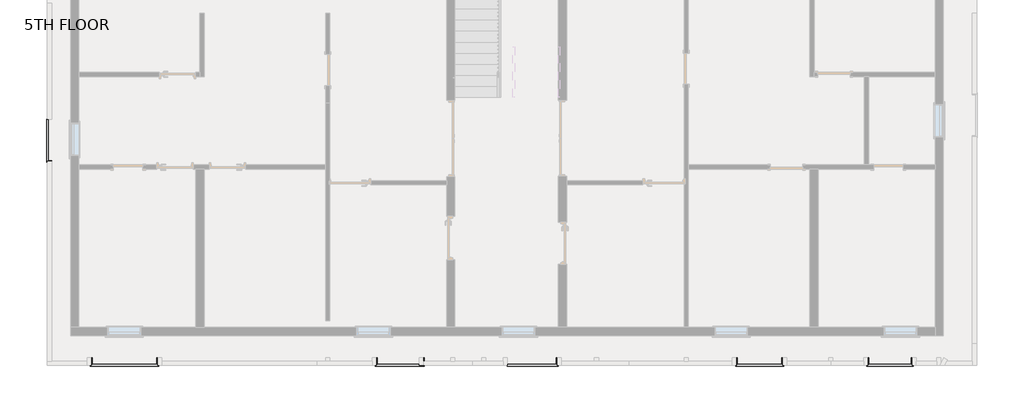
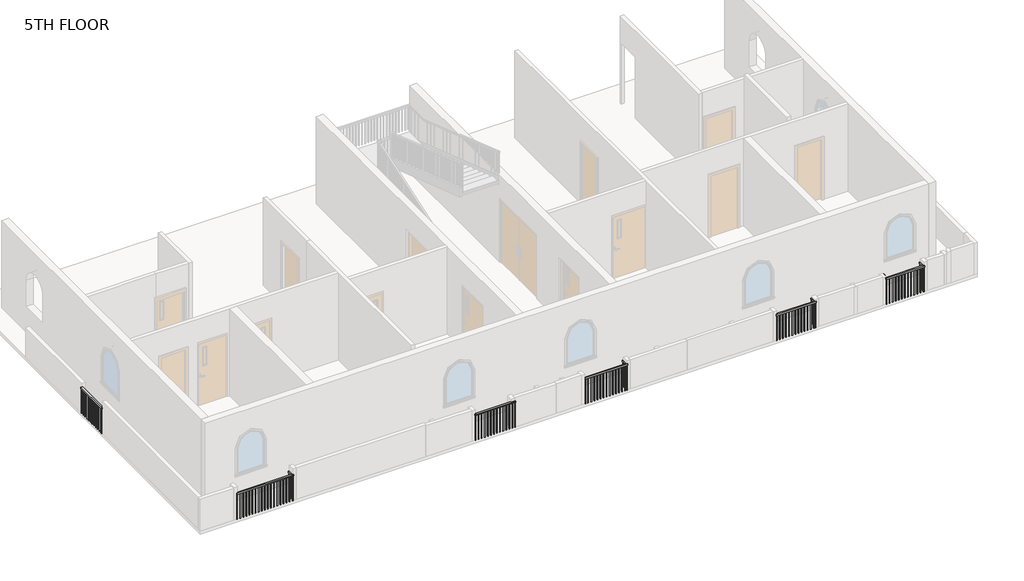
# One storey, part 3 of 7: 6 railings.
"""IFC4 building model written with IfcOpenShell, lengths in millimetres."""

from ifc_helpers import new_model, si_unit, frame, origin, place, context, project, spatial, polyline, outline, extrude, faceted_brep, element, save

model = new_model("IFC4")

# Units and contexts
model_context = context("Model", 3, world=origin())
ifc_project = project(units=[si_unit("LENGTHUNIT", "METRE", prefix="MILLI")], contexts=[model_context])

# Site, building, storey
site = spatial("IfcSite", under=ifc_project)
building = spatial("IfcBuilding", under=site)
storey = spatial("IfcBuildingStorey", under=building, Name="5TH FLOOR", Elevation=16002.0)

# Railings
placement = place(None, origin())
element("IfcRailing", 1, ObjectType="Handrail - Rectangular", at=placement, inside=storey, context=model_context, shape_type="SolidModel", body=[
    faceted_brep([(-11856.9067989, -4623.6932193, 16916.4), (-11856.9067989, -4623.6932193, 16865.6), (-11907.7067989, -4623.6932193, 16865.6), (-11907.7067989, -4623.6932193, 16916.4), (-11856.9067989, -4801.4932661, 16916.4), (-11856.9067989, -4801.4932661, 16865.6), (-11907.7067989, -4852.2932661, 16865.6), (-11907.7067989, -4852.2932661, 16916.4), (-10071.3470335, -4801.4932661, 16916.4), (-10071.3470335, -4801.4932661, 16865.6), (-10020.5470335, -4852.2932661, 16865.6), (-10020.5470335, -4852.2932661, 16916.4), (-10071.3470335, -4623.6932193, 16916.4), (-10020.5470335, -4623.6932193, 16916.4), (-10020.5470335, -4623.6932193, 16865.6), (-10071.3470335, -4623.6932193, 16865.6)], [[[0, 1, 2, 3]], [[1, 0, 4, 5]], [[2, 1, 5, 6]], [[3, 2, 6, 7]], [[0, 3, 7, 4]], [[5, 4, 8, 9]], [[6, 5, 9, 10]], [[7, 6, 10, 11]], [[4, 7, 11, 8]], [[12, 13, 14, 15]], [[9, 8, 12, 15]], [[10, 9, 15, 14]], [[11, 10, 14, 13]], [[8, 11, 13, 12]]]),
    extrude(outline(polyline([(-10036.4220335, -4633.2182661), (-10055.4720335, -4633.2182661), (-10055.4720335, -4614.1682661), (-10036.4220335, -4614.1682661), (-10036.4220335, -4633.2182661)])), frame((0.0, 0.0, 16002.0), z_axis=(0.0, 0.0, 1.0), x_axis=(1.0, 0.0, 0.0)), (0.0, 0.0, 1.0), 863.6),
    extrude(outline(polyline([(-10036.4220335, -4734.8182661), (-10055.4720335, -4734.8182661), (-10055.4720335, -4715.7682661), (-10036.4220335, -4715.7682661), (-10036.4220335, -4734.8182661)])), frame((0.0, 0.0, 16002.0), z_axis=(0.0, 0.0, 1.0), x_axis=(1.0, 0.0, 0.0)), (0.0, 0.0, 1.0), 863.6),
    extrude(outline(polyline([(-10063.0317989, -4836.4182661), (-10063.0317989, -4817.3682661), (-10043.9817989, -4817.3682661), (-10043.9817989, -4836.4182661), (-10063.0317989, -4836.4182661)])), frame((0.0, 0.0, 16002.0), z_axis=(0.0, 0.0, 1.0), x_axis=(1.0, 0.0, 0.0)), (0.0, 0.0, 1.0), 863.6),
    extrude(outline(polyline([(-10164.6317989, -4836.4182661), (-10164.6317989, -4817.3682661), (-10145.5817989, -4817.3682661), (-10145.5817989, -4836.4182661), (-10164.6317989, -4836.4182661)])), frame((0.0, 0.0, 16002.0), z_axis=(0.0, 0.0, 1.0), x_axis=(1.0, 0.0, 0.0)), (0.0, 0.0, 1.0), 863.6),
    extrude(outline(polyline([(-10266.2317989, -4836.4182661), (-10266.2317989, -4817.3682661), (-10247.1817989, -4817.3682661), (-10247.1817989, -4836.4182661), (-10266.2317989, -4836.4182661)])), frame((0.0, 0.0, 16002.0), z_axis=(0.0, 0.0, 1.0), x_axis=(1.0, 0.0, 0.0)), (0.0, 0.0, 1.0), 863.6),
    extrude(outline(polyline([(-10367.8317989, -4836.4182661), (-10367.8317989, -4817.3682661), (-10348.7817989, -4817.3682661), (-10348.7817989, -4836.4182661), (-10367.8317989, -4836.4182661)])), frame((0.0, 0.0, 16002.0), z_axis=(0.0, 0.0, 1.0), x_axis=(1.0, 0.0, 0.0)), (0.0, 0.0, 1.0), 863.6),
    extrude(outline(polyline([(-10469.4317989, -4836.4182661), (-10469.4317989, -4817.3682661), (-10450.3817989, -4817.3682661), (-10450.3817989, -4836.4182661), (-10469.4317989, -4836.4182661)])), frame((0.0, 0.0, 16002.0), z_axis=(0.0, 0.0, 1.0), x_axis=(1.0, 0.0, 0.0)), (0.0, 0.0, 1.0), 863.6),
    extrude(outline(polyline([(-10571.0317989, -4836.4182661), (-10571.0317989, -4817.3682661), (-10551.9817989, -4817.3682661), (-10551.9817989, -4836.4182661), (-10571.0317989, -4836.4182661)])), frame((0.0, 0.0, 16002.0), z_axis=(0.0, 0.0, 1.0), x_axis=(1.0, 0.0, 0.0)), (0.0, 0.0, 1.0), 863.6),
    extrude(outline(polyline([(-10672.6317989, -4836.4182661), (-10672.6317989, -4817.3682661), (-10653.5817989, -4817.3682661), (-10653.5817989, -4836.4182661), (-10672.6317989, -4836.4182661)])), frame((0.0, 0.0, 16002.0), z_axis=(0.0, 0.0, 1.0), x_axis=(1.0, 0.0, 0.0)), (0.0, 0.0, 1.0), 863.6),
    extrude(outline(polyline([(-10774.2317989, -4836.4182661), (-10774.2317989, -4817.3682661), (-10755.1817989, -4817.3682661), (-10755.1817989, -4836.4182661), (-10774.2317989, -4836.4182661)])), frame((0.0, 0.0, 16002.0), z_axis=(0.0, 0.0, 1.0), x_axis=(1.0, 0.0, 0.0)), (0.0, 0.0, 1.0), 863.6),
    extrude(outline(polyline([(-10875.8317989, -4836.4182661), (-10875.8317989, -4817.3682661), (-10856.7817989, -4817.3682661), (-10856.7817989, -4836.4182661), (-10875.8317989, -4836.4182661)])), frame((0.0, 0.0, 16002.0), z_axis=(0.0, 0.0, 1.0), x_axis=(1.0, 0.0, 0.0)), (0.0, 0.0, 1.0), 863.6),
    extrude(outline(polyline([(-10977.4317989, -4836.4182661), (-10977.4317989, -4817.3682661), (-10958.3817989, -4817.3682661), (-10958.3817989, -4836.4182661), (-10977.4317989, -4836.4182661)])), frame((0.0, 0.0, 16002.0), z_axis=(0.0, 0.0, 1.0), x_axis=(1.0, 0.0, 0.0)), (0.0, 0.0, 1.0), 863.6),
    extrude(outline(polyline([(-11079.0317989, -4836.4182661), (-11079.0317989, -4817.3682661), (-11059.9817989, -4817.3682661), (-11059.9817989, -4836.4182661), (-11079.0317989, -4836.4182661)])), frame((0.0, 0.0, 16002.0), z_axis=(0.0, 0.0, 1.0), x_axis=(1.0, 0.0, 0.0)), (0.0, 0.0, 1.0), 863.6),
    extrude(outline(polyline([(-11180.6317989, -4836.4182661), (-11180.6317989, -4817.3682661), (-11161.5817989, -4817.3682661), (-11161.5817989, -4836.4182661), (-11180.6317989, -4836.4182661)])), frame((0.0, 0.0, 16002.0), z_axis=(0.0, 0.0, 1.0), x_axis=(1.0, 0.0, 0.0)), (0.0, 0.0, 1.0), 863.6),
    extrude(outline(polyline([(-11282.2317989, -4836.4182661), (-11282.2317989, -4817.3682661), (-11263.1817989, -4817.3682661), (-11263.1817989, -4836.4182661), (-11282.2317989, -4836.4182661)])), frame((0.0, 0.0, 16002.0), z_axis=(0.0, 0.0, 1.0), x_axis=(1.0, 0.0, 0.0)), (0.0, 0.0, 1.0), 863.6),
    extrude(outline(polyline([(-11383.8317989, -4836.4182661), (-11383.8317989, -4817.3682661), (-11364.7817989, -4817.3682661), (-11364.7817989, -4836.4182661), (-11383.8317989, -4836.4182661)])), frame((0.0, 0.0, 16002.0), z_axis=(0.0, 0.0, 1.0), x_axis=(1.0, 0.0, 0.0)), (0.0, 0.0, 1.0), 863.6),
    extrude(outline(polyline([(-11485.4317989, -4836.4182661), (-11485.4317989, -4817.3682661), (-11466.3817989, -4817.3682661), (-11466.3817989, -4836.4182661), (-11485.4317989, -4836.4182661)])), frame((0.0, 0.0, 16002.0), z_axis=(0.0, 0.0, 1.0), x_axis=(1.0, 0.0, 0.0)), (0.0, 0.0, 1.0), 863.6),
    extrude(outline(polyline([(-11587.0317989, -4836.4182661), (-11587.0317989, -4817.3682661), (-11567.9817989, -4817.3682661), (-11567.9817989, -4836.4182661), (-11587.0317989, -4836.4182661)])), frame((0.0, 0.0, 16002.0), z_axis=(0.0, 0.0, 1.0), x_axis=(1.0, 0.0, 0.0)), (0.0, 0.0, 1.0), 863.6),
    extrude(outline(polyline([(-11688.6317989, -4836.4182661), (-11688.6317989, -4817.3682661), (-11669.5817989, -4817.3682661), (-11669.5817989, -4836.4182661), (-11688.6317989, -4836.4182661)])), frame((0.0, 0.0, 16002.0), z_axis=(0.0, 0.0, 1.0), x_axis=(1.0, 0.0, 0.0)), (0.0, 0.0, 1.0), 863.6),
    extrude(outline(polyline([(-11790.2317989, -4836.4182661), (-11790.2317989, -4817.3682661), (-11771.1817989, -4817.3682661), (-11771.1817989, -4836.4182661), (-11790.2317989, -4836.4182661)])), frame((0.0, 0.0, 16002.0), z_axis=(0.0, 0.0, 1.0), x_axis=(1.0, 0.0, 0.0)), (0.0, 0.0, 1.0), 863.6),
    extrude(outline(polyline([(-11891.8317989, -4817.3682193), (-11872.7817989, -4817.3682193), (-11872.7817989, -4836.4182193), (-11891.8317989, -4836.4182193), (-11891.8317989, -4817.3682193)])), frame((0.0, 0.0, 16002.0), z_axis=(0.0, 0.0, 1.0), x_axis=(1.0, 0.0, 0.0)), (0.0, 0.0, 1.0), 863.6),
    extrude(outline(polyline([(-11891.8317989, -4715.7682193), (-11872.7817989, -4715.7682193), (-11872.7817989, -4734.8182193), (-11891.8317989, -4734.8182193), (-11891.8317989, -4715.7682193)])), frame((0.0, 0.0, 16002.0), z_axis=(0.0, 0.0, 1.0), x_axis=(1.0, 0.0, 0.0)), (0.0, 0.0, 1.0), 863.6),
    extrude(outline(polyline([(-10055.4720335, -4836.4182661), (-10055.4720335, -4817.3682661), (-10036.4220335, -4817.3682661), (-10036.4220335, -4836.4182661), (-10055.4720335, -4836.4182661)])), frame((0.0, 0.0, 16002.0), z_axis=(0.0, 0.0, 1.0), x_axis=(1.0, 0.0, 0.0)), (0.0, 0.0, 1.0), 863.6),
    extrude(outline(polyline([(-11891.8317989, -4817.3682661), (-11872.7817989, -4817.3682661), (-11872.7817989, -4836.4182661), (-11891.8317989, -4836.4182661), (-11891.8317989, -4817.3682661)])), frame((0.0, 0.0, 16002.0), z_axis=(0.0, 0.0, 1.0), x_axis=(1.0, 0.0, 0.0)), (0.0, 0.0, 1.0), 863.6),
    extrude(outline(polyline([(-10036.4220335, -4642.7432193), (-10055.4720335, -4642.7432193), (-10055.4720335, -4623.6932193), (-10036.4220335, -4623.6932193), (-10036.4220335, -4642.7432193)])), frame((0.0, 0.0, 16002.0), z_axis=(0.0, 0.0, 1.0), x_axis=(1.0, 0.0, 0.0)), (0.0, 0.0, 1.0), 863.6),
    extrude(outline(polyline([(-11891.8317989, -4623.6932193), (-11872.7817989, -4623.6932193), (-11872.7817989, -4642.7432193), (-11891.8317989, -4642.7432193), (-11891.8317989, -4623.6932193)])), frame((0.0, 0.0, 16002.0), z_axis=(0.0, 0.0, 1.0), x_axis=(1.0, 0.0, 0.0)), (0.0, 0.0, 1.0), 863.6),
])
element("IfcRailing", 2, ObjectType="Handrail - Rectangular", at=placement, inside=storey, context=model_context, shape_type="SolidModel", body=[
    faceted_brep([(-3995.0987995, -4623.6932193, 16916.4), (-3995.0987995, -4623.6932193, 16865.6), (-4045.8987995, -4623.6932193, 16865.6), (-4045.8987995, -4623.6932193, 16916.4), (-3995.0987995, -4801.4932661, 16916.4), (-3995.0987995, -4801.4932661, 16865.6), (-4045.8987995, -4852.2932661, 16865.6), (-4045.8987995, -4852.2932661, 16916.4), (-2750.4987995, -4801.4932661, 16916.4), (-2750.4987995, -4801.4932661, 16865.6), (-2699.6987995, -4852.2932661, 16865.6), (-2699.6987995, -4852.2932661, 16916.4), (-2750.4987995, -4623.6932193, 16916.4), (-2699.6987995, -4623.6932193, 16916.4), (-2699.6987995, -4623.6932193, 16865.6), (-2750.4987995, -4623.6932193, 16865.6)], [[[0, 1, 2, 3]], [[1, 0, 4, 5]], [[2, 1, 5, 6]], [[3, 2, 6, 7]], [[0, 3, 7, 4]], [[5, 4, 8, 9]], [[6, 5, 9, 10]], [[7, 6, 10, 11]], [[4, 7, 11, 8]], [[12, 13, 14, 15]], [[9, 8, 12, 15]], [[10, 9, 15, 14]], [[11, 10, 14, 13]], [[8, 11, 13, 12]]]),
    extrude(outline(polyline([(-2715.5737995, -4633.2182661), (-2734.6237995, -4633.2182661), (-2734.6237995, -4614.1682661), (-2715.5737995, -4614.1682661), (-2715.5737995, -4633.2182661)])), frame((0.0, 0.0, 16002.0), z_axis=(0.0, 0.0, 1.0), x_axis=(1.0, 0.0, 0.0)), (0.0, 0.0, 1.0), 863.6),
    extrude(outline(polyline([(-2715.5737995, -4734.8182661), (-2734.6237995, -4734.8182661), (-2734.6237995, -4715.7682661), (-2715.5737995, -4715.7682661), (-2715.5737995, -4734.8182661)])), frame((0.0, 0.0, 16002.0), z_axis=(0.0, 0.0, 1.0), x_axis=(1.0, 0.0, 0.0)), (0.0, 0.0, 1.0), 863.6),
    extrude(outline(polyline([(-2810.8237995, -4836.4182661), (-2810.8237995, -4817.3682661), (-2791.7737995, -4817.3682661), (-2791.7737995, -4836.4182661), (-2810.8237995, -4836.4182661)])), frame((0.0, 0.0, 16002.0), z_axis=(0.0, 0.0, 1.0), x_axis=(1.0, 0.0, 0.0)), (0.0, 0.0, 1.0), 863.6),
    extrude(outline(polyline([(-2912.4237995, -4836.4182661), (-2912.4237995, -4817.3682661), (-2893.3737995, -4817.3682661), (-2893.3737995, -4836.4182661), (-2912.4237995, -4836.4182661)])), frame((0.0, 0.0, 16002.0), z_axis=(0.0, 0.0, 1.0), x_axis=(1.0, 0.0, 0.0)), (0.0, 0.0, 1.0), 863.6),
    extrude(outline(polyline([(-3014.0237995, -4836.4182661), (-3014.0237995, -4817.3682661), (-2994.9737995, -4817.3682661), (-2994.9737995, -4836.4182661), (-3014.0237995, -4836.4182661)])), frame((0.0, 0.0, 16002.0), z_axis=(0.0, 0.0, 1.0), x_axis=(1.0, 0.0, 0.0)), (0.0, 0.0, 1.0), 863.6),
    extrude(outline(polyline([(-3115.6237995, -4836.4182661), (-3115.6237995, -4817.3682661), (-3096.5737995, -4817.3682661), (-3096.5737995, -4836.4182661), (-3115.6237995, -4836.4182661)])), frame((0.0, 0.0, 16002.0), z_axis=(0.0, 0.0, 1.0), x_axis=(1.0, 0.0, 0.0)), (0.0, 0.0, 1.0), 863.6),
    extrude(outline(polyline([(-3217.2237995, -4836.4182661), (-3217.2237995, -4817.3682661), (-3198.1737995, -4817.3682661), (-3198.1737995, -4836.4182661), (-3217.2237995, -4836.4182661)])), frame((0.0, 0.0, 16002.0), z_axis=(0.0, 0.0, 1.0), x_axis=(1.0, 0.0, 0.0)), (0.0, 0.0, 1.0), 863.6),
    extrude(outline(polyline([(-3318.8237995, -4836.4182661), (-3318.8237995, -4817.3682661), (-3299.7737995, -4817.3682661), (-3299.7737995, -4836.4182661), (-3318.8237995, -4836.4182661)])), frame((0.0, 0.0, 16002.0), z_axis=(0.0, 0.0, 1.0), x_axis=(1.0, 0.0, 0.0)), (0.0, 0.0, 1.0), 863.6),
    extrude(outline(polyline([(-3420.4237995, -4836.4182661), (-3420.4237995, -4817.3682661), (-3401.3737995, -4817.3682661), (-3401.3737995, -4836.4182661), (-3420.4237995, -4836.4182661)])), frame((0.0, 0.0, 16002.0), z_axis=(0.0, 0.0, 1.0), x_axis=(1.0, 0.0, 0.0)), (0.0, 0.0, 1.0), 863.6),
    extrude(outline(polyline([(-3522.0237995, -4836.4182661), (-3522.0237995, -4817.3682661), (-3502.9737995, -4817.3682661), (-3502.9737995, -4836.4182661), (-3522.0237995, -4836.4182661)])), frame((0.0, 0.0, 16002.0), z_axis=(0.0, 0.0, 1.0), x_axis=(1.0, 0.0, 0.0)), (0.0, 0.0, 1.0), 863.6),
    extrude(outline(polyline([(-3623.6237995, -4836.4182661), (-3623.6237995, -4817.3682661), (-3604.5737995, -4817.3682661), (-3604.5737995, -4836.4182661), (-3623.6237995, -4836.4182661)])), frame((0.0, 0.0, 16002.0), z_axis=(0.0, 0.0, 1.0), x_axis=(1.0, 0.0, 0.0)), (0.0, 0.0, 1.0), 863.6),
    extrude(outline(polyline([(-3725.2237995, -4836.4182661), (-3725.2237995, -4817.3682661), (-3706.1737995, -4817.3682661), (-3706.1737995, -4836.4182661), (-3725.2237995, -4836.4182661)])), frame((0.0, 0.0, 16002.0), z_axis=(0.0, 0.0, 1.0), x_axis=(1.0, 0.0, 0.0)), (0.0, 0.0, 1.0), 863.6),
    extrude(outline(polyline([(-3826.8237995, -4836.4182661), (-3826.8237995, -4817.3682661), (-3807.7737995, -4817.3682661), (-3807.7737995, -4836.4182661), (-3826.8237995, -4836.4182661)])), frame((0.0, 0.0, 16002.0), z_axis=(0.0, 0.0, 1.0), x_axis=(1.0, 0.0, 0.0)), (0.0, 0.0, 1.0), 863.6),
    extrude(outline(polyline([(-3928.4237995, -4836.4182661), (-3928.4237995, -4817.3682661), (-3909.3737995, -4817.3682661), (-3909.3737995, -4836.4182661), (-3928.4237995, -4836.4182661)])), frame((0.0, 0.0, 16002.0), z_axis=(0.0, 0.0, 1.0), x_axis=(1.0, 0.0, 0.0)), (0.0, 0.0, 1.0), 863.6),
    extrude(outline(polyline([(-4030.0237995, -4817.3682193), (-4010.9737995, -4817.3682193), (-4010.9737995, -4836.4182193), (-4030.0237995, -4836.4182193), (-4030.0237995, -4817.3682193)])), frame((0.0, 0.0, 16002.0), z_axis=(0.0, 0.0, 1.0), x_axis=(1.0, 0.0, 0.0)), (0.0, 0.0, 1.0), 863.6),
    extrude(outline(polyline([(-4030.0237995, -4715.7682193), (-4010.9737995, -4715.7682193), (-4010.9737995, -4734.8182193), (-4030.0237995, -4734.8182193), (-4030.0237995, -4715.7682193)])), frame((0.0, 0.0, 16002.0), z_axis=(0.0, 0.0, 1.0), x_axis=(1.0, 0.0, 0.0)), (0.0, 0.0, 1.0), 863.6),
    extrude(outline(polyline([(-2734.6237995, -4836.4182661), (-2734.6237995, -4817.3682661), (-2715.5737995, -4817.3682661), (-2715.5737995, -4836.4182661), (-2734.6237995, -4836.4182661)])), frame((0.0, 0.0, 16002.0), z_axis=(0.0, 0.0, 1.0), x_axis=(1.0, 0.0, 0.0)), (0.0, 0.0, 1.0), 863.6),
    extrude(outline(polyline([(-4030.0237995, -4817.3682661), (-4010.9737995, -4817.3682661), (-4010.9737995, -4836.4182661), (-4030.0237995, -4836.4182661), (-4030.0237995, -4817.3682661)])), frame((0.0, 0.0, 16002.0), z_axis=(0.0, 0.0, 1.0), x_axis=(1.0, 0.0, 0.0)), (0.0, 0.0, 1.0), 863.6),
    extrude(outline(polyline([(-2715.5737995, -4642.7432193), (-2734.6237995, -4642.7432193), (-2734.6237995, -4623.6932193), (-2715.5737995, -4623.6932193), (-2715.5737995, -4642.7432193)])), frame((0.0, 0.0, 16002.0), z_axis=(0.0, 0.0, 1.0), x_axis=(1.0, 0.0, 0.0)), (0.0, 0.0, 1.0), 863.6),
    extrude(outline(polyline([(-4030.0237995, -4623.6932193), (-4010.9737995, -4623.6932193), (-4010.9737995, -4642.7432193), (-4030.0237995, -4642.7432193), (-4030.0237995, -4623.6932193)])), frame((0.0, 0.0, 16002.0), z_axis=(0.0, 0.0, 1.0), x_axis=(1.0, 0.0, 0.0)), (0.0, 0.0, 1.0), 863.6),
])
element("IfcRailing", 3, ObjectType="Handrail - Rectangular", at=placement, inside=storey, context=model_context, shape_type="SolidModel", body=[
    faceted_brep([(-406.2065315, -4801.4932661, 16916.4), (-406.2065315, -4801.4932661, 16865.6), (-406.2065315, -4852.2932661, 16865.6), (-406.2065315, -4852.2932661, 16916.4), (944.6932011, -4801.4932661, 16916.4), (944.6932011, -4801.4932661, 16865.6), (995.4932011, -4852.2932661, 16865.6), (995.4932011, -4852.2932661, 16916.4), (944.6932011, -4623.6932193, 16916.4), (995.4932011, -4623.6932193, 16916.4), (995.4932011, -4623.6932193, 16865.6), (944.6932011, -4623.6932193, 16865.6)], [[[0, 1, 2, 3]], [[1, 0, 4, 5]], [[2, 1, 5, 6]], [[3, 2, 6, 7]], [[0, 3, 7, 4]], [[8, 9, 10, 11]], [[5, 4, 8, 11]], [[6, 5, 11, 10]], [[7, 6, 10, 9]], [[4, 7, 9, 8]]]),
    extrude(outline(polyline([(979.6182011, -4633.2182661), (960.5682011, -4633.2182661), (960.5682011, -4614.1682661), (979.6182011, -4614.1682661), (979.6182011, -4633.2182661)])), frame((0.0, 0.0, 16002.0), z_axis=(0.0, 0.0, 1.0), x_axis=(1.0, 0.0, 0.0)), (0.0, 0.0, 1.0), 863.6),
    extrude(outline(polyline([(979.6182011, -4734.8182661), (960.5682011, -4734.8182661), (960.5682011, -4715.7682661), (979.6182011, -4715.7682661), (979.6182011, -4734.8182661)])), frame((0.0, 0.0, 16002.0), z_axis=(0.0, 0.0, 1.0), x_axis=(1.0, 0.0, 0.0)), (0.0, 0.0, 1.0), 863.6),
    extrude(outline(polyline([(905.0684685, -4836.4182661), (905.0684685, -4817.3682661), (924.1184685, -4817.3682661), (924.1184685, -4836.4182661), (905.0684685, -4836.4182661)])), frame((0.0, 0.0, 16002.0), z_axis=(0.0, 0.0, 1.0), x_axis=(1.0, 0.0, 0.0)), (0.0, 0.0, 1.0), 863.6),
    extrude(outline(polyline([(803.4684685, -4836.4182661), (803.4684685, -4817.3682661), (822.5184685, -4817.3682661), (822.5184685, -4836.4182661), (803.4684685, -4836.4182661)])), frame((0.0, 0.0, 16002.0), z_axis=(0.0, 0.0, 1.0), x_axis=(1.0, 0.0, 0.0)), (0.0, 0.0, 1.0), 863.6),
    extrude(outline(polyline([(701.8684685, -4836.4182661), (701.8684685, -4817.3682661), (720.9184685, -4817.3682661), (720.9184685, -4836.4182661), (701.8684685, -4836.4182661)])), frame((0.0, 0.0, 16002.0), z_axis=(0.0, 0.0, 1.0), x_axis=(1.0, 0.0, 0.0)), (0.0, 0.0, 1.0), 863.6),
    extrude(outline(polyline([(600.2684685, -4836.4182661), (600.2684685, -4817.3682661), (619.3184685, -4817.3682661), (619.3184685, -4836.4182661), (600.2684685, -4836.4182661)])), frame((0.0, 0.0, 16002.0), z_axis=(0.0, 0.0, 1.0), x_axis=(1.0, 0.0, 0.0)), (0.0, 0.0, 1.0), 863.6),
    extrude(outline(polyline([(498.6684685, -4836.4182661), (498.6684685, -4817.3682661), (517.7184685, -4817.3682661), (517.7184685, -4836.4182661), (498.6684685, -4836.4182661)])), frame((0.0, 0.0, 16002.0), z_axis=(0.0, 0.0, 1.0), x_axis=(1.0, 0.0, 0.0)), (0.0, 0.0, 1.0), 863.6),
    extrude(outline(polyline([(397.0684685, -4836.4182661), (397.0684685, -4817.3682661), (416.1184685, -4817.3682661), (416.1184685, -4836.4182661), (397.0684685, -4836.4182661)])), frame((0.0, 0.0, 16002.0), z_axis=(0.0, 0.0, 1.0), x_axis=(1.0, 0.0, 0.0)), (0.0, 0.0, 1.0), 863.6),
    extrude(outline(polyline([(295.4684685, -4836.4182661), (295.4684685, -4817.3682661), (314.5184685, -4817.3682661), (314.5184685, -4836.4182661), (295.4684685, -4836.4182661)])), frame((0.0, 0.0, 16002.0), z_axis=(0.0, 0.0, 1.0), x_axis=(1.0, 0.0, 0.0)), (0.0, 0.0, 1.0), 863.6),
    extrude(outline(polyline([(193.8684685, -4836.4182661), (193.8684685, -4817.3682661), (212.9184685, -4817.3682661), (212.9184685, -4836.4182661), (193.8684685, -4836.4182661)])), frame((0.0, 0.0, 16002.0), z_axis=(0.0, 0.0, 1.0), x_axis=(1.0, 0.0, 0.0)), (0.0, 0.0, 1.0), 863.6),
    extrude(outline(polyline([(92.2684685, -4836.4182661), (92.2684685, -4817.3682661), (111.3184685, -4817.3682661), (111.3184685, -4836.4182661), (92.2684685, -4836.4182661)])), frame((0.0, 0.0, 16002.0), z_axis=(0.0, 0.0, 1.0), x_axis=(1.0, 0.0, 0.0)), (0.0, 0.0, 1.0), 863.6),
    extrude(outline(polyline([(-9.3315315, -4836.4182661), (-9.3315315, -4817.3682661), (9.7184685, -4817.3682661), (9.7184685, -4836.4182661), (-9.3315315, -4836.4182661)])), frame((0.0, 0.0, 16002.0), z_axis=(0.0, 0.0, 1.0), x_axis=(1.0, 0.0, 0.0)), (0.0, 0.0, 1.0), 863.6),
    extrude(outline(polyline([(-110.9315315, -4836.4182661), (-110.9315315, -4817.3682661), (-91.8815315, -4817.3682661), (-91.8815315, -4836.4182661), (-110.9315315, -4836.4182661)])), frame((0.0, 0.0, 16002.0), z_axis=(0.0, 0.0, 1.0), x_axis=(1.0, 0.0, 0.0)), (0.0, 0.0, 1.0), 863.6),
    extrude(outline(polyline([(-212.5315315, -4836.4182661), (-212.5315315, -4817.3682661), (-193.4815315, -4817.3682661), (-193.4815315, -4836.4182661), (-212.5315315, -4836.4182661)])), frame((0.0, 0.0, 16002.0), z_axis=(0.0, 0.0, 1.0), x_axis=(1.0, 0.0, 0.0)), (0.0, 0.0, 1.0), 863.6),
    extrude(outline(polyline([(-314.1315315, -4836.4182661), (-314.1315315, -4817.3682661), (-295.0815315, -4817.3682661), (-295.0815315, -4836.4182661), (-314.1315315, -4836.4182661)])), frame((0.0, 0.0, 16002.0), z_axis=(0.0, 0.0, 1.0), x_axis=(1.0, 0.0, 0.0)), (0.0, 0.0, 1.0), 863.6),
    extrude(outline(polyline([(960.5682011, -4836.4182661), (960.5682011, -4817.3682661), (979.6182011, -4817.3682661), (979.6182011, -4836.4182661), (960.5682011, -4836.4182661)])), frame((0.0, 0.0, 16002.0), z_axis=(0.0, 0.0, 1.0), x_axis=(1.0, 0.0, 0.0)), (0.0, 0.0, 1.0), 863.6),
    extrude(outline(polyline([(979.6182011, -4642.7432193), (960.5682011, -4642.7432193), (960.5682011, -4623.6932193), (979.6182011, -4623.6932193), (979.6182011, -4642.7432193)])), frame((0.0, 0.0, 16002.0), z_axis=(0.0, 0.0, 1.0), x_axis=(1.0, 0.0, 0.0)), (0.0, 0.0, 1.0), 863.6),
    extrude(outline(polyline([(-406.2065315, -4836.4182661), (-406.2065315, -4817.3682661), (-387.1565315, -4817.3682661), (-387.1565315, -4836.4182661), (-406.2065315, -4836.4182661)])), frame((0.0, 0.0, 16002.0), z_axis=(0.0, 0.0, 1.0), x_axis=(1.0, 0.0, 0.0)), (0.0, 0.0, 1.0), 863.6),
])
element("IfcRailing", 4, ObjectType="Handrail - Rectangular", at=placement, inside=storey, context=model_context, shape_type="SolidModel", body=[
    faceted_brep([(5942.6512082, -4623.6932193, 16916.4), (5942.6512082, -4623.6932193, 16865.6), (5891.8512082, -4623.6932193, 16865.6), (5891.8512082, -4623.6932193, 16916.4), (5942.6512082, -4801.4932661, 16916.4), (5942.6512082, -4801.4932661, 16865.6), (5891.8512082, -4852.2932661, 16865.6), (5891.8512082, -4852.2932661, 16916.4), (7164.9011643, -4801.4932661, 16916.4), (7164.9011643, -4801.4932661, 16865.6), (7215.7011643, -4852.2932661, 16865.6), (7215.7011643, -4852.2932661, 16916.4), (7164.9011643, -4623.6932193, 16916.4), (7215.7011643, -4623.6932193, 16916.4), (7215.7011643, -4623.6932193, 16865.6), (7164.9011643, -4623.6932193, 16865.6)], [[[0, 1, 2, 3]], [[1, 0, 4, 5]], [[2, 1, 5, 6]], [[3, 2, 6, 7]], [[0, 3, 7, 4]], [[5, 4, 8, 9]], [[6, 5, 9, 10]], [[7, 6, 10, 11]], [[4, 7, 11, 8]], [[12, 13, 14, 15]], [[9, 8, 12, 15]], [[10, 9, 15, 14]], [[11, 10, 14, 13]], [[8, 11, 13, 12]]]),
    extrude(outline(polyline([(7199.8261643, -4633.2182661), (7180.7761643, -4633.2182661), (7180.7761643, -4614.1682661), (7199.8261643, -4614.1682661), (7199.8261643, -4633.2182661)])), frame((0.0, 0.0, 16002.0), z_axis=(0.0, 0.0, 1.0), x_axis=(1.0, 0.0, 0.0)), (0.0, 0.0, 1.0), 863.6),
    extrude(outline(polyline([(7199.8261643, -4734.8182661), (7180.7761643, -4734.8182661), (7180.7761643, -4715.7682661), (7199.8261643, -4715.7682661), (7199.8261643, -4734.8182661)])), frame((0.0, 0.0, 16002.0), z_axis=(0.0, 0.0, 1.0), x_axis=(1.0, 0.0, 0.0)), (0.0, 0.0, 1.0), 863.6),
    extrude(outline(polyline([(7126.9262082, -4836.4182661), (7126.9262082, -4817.3682661), (7145.9762082, -4817.3682661), (7145.9762082, -4836.4182661), (7126.9262082, -4836.4182661)])), frame((0.0, 0.0, 16002.0), z_axis=(0.0, 0.0, 1.0), x_axis=(1.0, 0.0, 0.0)), (0.0, 0.0, 1.0), 863.6),
    extrude(outline(polyline([(7025.3262082, -4836.4182661), (7025.3262082, -4817.3682661), (7044.3762082, -4817.3682661), (7044.3762082, -4836.4182661), (7025.3262082, -4836.4182661)])), frame((0.0, 0.0, 16002.0), z_axis=(0.0, 0.0, 1.0), x_axis=(1.0, 0.0, 0.0)), (0.0, 0.0, 1.0), 863.6),
    extrude(outline(polyline([(6923.7262082, -4836.4182661), (6923.7262082, -4817.3682661), (6942.7762082, -4817.3682661), (6942.7762082, -4836.4182661), (6923.7262082, -4836.4182661)])), frame((0.0, 0.0, 16002.0), z_axis=(0.0, 0.0, 1.0), x_axis=(1.0, 0.0, 0.0)), (0.0, 0.0, 1.0), 863.6),
    extrude(outline(polyline([(6822.1262082, -4836.4182661), (6822.1262082, -4817.3682661), (6841.1762082, -4817.3682661), (6841.1762082, -4836.4182661), (6822.1262082, -4836.4182661)])), frame((0.0, 0.0, 16002.0), z_axis=(0.0, 0.0, 1.0), x_axis=(1.0, 0.0, 0.0)), (0.0, 0.0, 1.0), 863.6),
    extrude(outline(polyline([(6720.5262082, -4836.4182661), (6720.5262082, -4817.3682661), (6739.5762082, -4817.3682661), (6739.5762082, -4836.4182661), (6720.5262082, -4836.4182661)])), frame((0.0, 0.0, 16002.0), z_axis=(0.0, 0.0, 1.0), x_axis=(1.0, 0.0, 0.0)), (0.0, 0.0, 1.0), 863.6),
    extrude(outline(polyline([(6618.9262082, -4836.4182661), (6618.9262082, -4817.3682661), (6637.9762082, -4817.3682661), (6637.9762082, -4836.4182661), (6618.9262082, -4836.4182661)])), frame((0.0, 0.0, 16002.0), z_axis=(0.0, 0.0, 1.0), x_axis=(1.0, 0.0, 0.0)), (0.0, 0.0, 1.0), 863.6),
    extrude(outline(polyline([(6517.3262082, -4836.4182661), (6517.3262082, -4817.3682661), (6536.3762082, -4817.3682661), (6536.3762082, -4836.4182661), (6517.3262082, -4836.4182661)])), frame((0.0, 0.0, 16002.0), z_axis=(0.0, 0.0, 1.0), x_axis=(1.0, 0.0, 0.0)), (0.0, 0.0, 1.0), 863.6),
    extrude(outline(polyline([(6415.7262082, -4836.4182661), (6415.7262082, -4817.3682661), (6434.7762082, -4817.3682661), (6434.7762082, -4836.4182661), (6415.7262082, -4836.4182661)])), frame((0.0, 0.0, 16002.0), z_axis=(0.0, 0.0, 1.0), x_axis=(1.0, 0.0, 0.0)), (0.0, 0.0, 1.0), 863.6),
    extrude(outline(polyline([(6314.1262082, -4836.4182661), (6314.1262082, -4817.3682661), (6333.1762082, -4817.3682661), (6333.1762082, -4836.4182661), (6314.1262082, -4836.4182661)])), frame((0.0, 0.0, 16002.0), z_axis=(0.0, 0.0, 1.0), x_axis=(1.0, 0.0, 0.0)), (0.0, 0.0, 1.0), 863.6),
    extrude(outline(polyline([(6212.5262082, -4836.4182661), (6212.5262082, -4817.3682661), (6231.5762082, -4817.3682661), (6231.5762082, -4836.4182661), (6212.5262082, -4836.4182661)])), frame((0.0, 0.0, 16002.0), z_axis=(0.0, 0.0, 1.0), x_axis=(1.0, 0.0, 0.0)), (0.0, 0.0, 1.0), 863.6),
    extrude(outline(polyline([(6110.9262082, -4836.4182661), (6110.9262082, -4817.3682661), (6129.9762082, -4817.3682661), (6129.9762082, -4836.4182661), (6110.9262082, -4836.4182661)])), frame((0.0, 0.0, 16002.0), z_axis=(0.0, 0.0, 1.0), x_axis=(1.0, 0.0, 0.0)), (0.0, 0.0, 1.0), 863.6),
    extrude(outline(polyline([(6009.3262082, -4836.4182661), (6009.3262082, -4817.3682661), (6028.3762082, -4817.3682661), (6028.3762082, -4836.4182661), (6009.3262082, -4836.4182661)])), frame((0.0, 0.0, 16002.0), z_axis=(0.0, 0.0, 1.0), x_axis=(1.0, 0.0, 0.0)), (0.0, 0.0, 1.0), 863.6),
    extrude(outline(polyline([(5907.7262082, -4817.3682193), (5926.7762082, -4817.3682193), (5926.7762082, -4836.4182193), (5907.7262082, -4836.4182193), (5907.7262082, -4817.3682193)])), frame((0.0, 0.0, 16002.0), z_axis=(0.0, 0.0, 1.0), x_axis=(1.0, 0.0, 0.0)), (0.0, 0.0, 1.0), 863.6),
    extrude(outline(polyline([(5907.7262082, -4715.7682193), (5926.7762082, -4715.7682193), (5926.7762082, -4734.8182193), (5907.7262082, -4734.8182193), (5907.7262082, -4715.7682193)])), frame((0.0, 0.0, 16002.0), z_axis=(0.0, 0.0, 1.0), x_axis=(1.0, 0.0, 0.0)), (0.0, 0.0, 1.0), 863.6),
    extrude(outline(polyline([(7180.7761643, -4836.4182661), (7180.7761643, -4817.3682661), (7199.8261643, -4817.3682661), (7199.8261643, -4836.4182661), (7180.7761643, -4836.4182661)])), frame((0.0, 0.0, 16002.0), z_axis=(0.0, 0.0, 1.0), x_axis=(1.0, 0.0, 0.0)), (0.0, 0.0, 1.0), 863.6),
    extrude(outline(polyline([(5907.7262082, -4817.3682661), (5926.7762082, -4817.3682661), (5926.7762082, -4836.4182661), (5907.7262082, -4836.4182661), (5907.7262082, -4817.3682661)])), frame((0.0, 0.0, 16002.0), z_axis=(0.0, 0.0, 1.0), x_axis=(1.0, 0.0, 0.0)), (0.0, 0.0, 1.0), 863.6),
    extrude(outline(polyline([(7199.8261643, -4642.7432193), (7180.7761643, -4642.7432193), (7180.7761643, -4623.6932193), (7199.8261643, -4623.6932193), (7199.8261643, -4642.7432193)])), frame((0.0, 0.0, 16002.0), z_axis=(0.0, 0.0, 1.0), x_axis=(1.0, 0.0, 0.0)), (0.0, 0.0, 1.0), 863.6),
    extrude(outline(polyline([(5907.7262082, -4623.6932193), (5926.7762082, -4623.6932193), (5926.7762082, -4642.7432193), (5907.7262082, -4642.7432193), (5907.7262082, -4623.6932193)])), frame((0.0, 0.0, 16002.0), z_axis=(0.0, 0.0, 1.0), x_axis=(1.0, 0.0, 0.0)), (0.0, 0.0, 1.0), 863.6),
])
element("IfcRailing", 5, ObjectType="Handrail - Rectangular", at=placement, inside=storey, context=model_context, shape_type="SolidModel", body=[
    faceted_brep([(9562.1512082, -4623.6932193, 16916.4), (9562.1512082, -4623.6932193, 16865.6), (9511.3512082, -4623.6932193, 16865.6), (9511.3512082, -4623.6932193, 16916.4), (9562.1512082, -4801.4932661, 16916.4), (9562.1512082, -4801.4932661, 16865.6), (9511.3512082, -4852.2932661, 16865.6), (9511.3512082, -4852.2932661, 16916.4), (10738.7617205, -4801.4932661, 16916.4), (10738.7617205, -4801.4932661, 16865.6), (10789.5617205, -4852.2932661, 16865.6), (10789.5617205, -4852.2932661, 16916.4), (10738.7617205, -4623.6932193, 16916.4), (10789.5617205, -4623.6932193, 16916.4), (10789.5617205, -4623.6932193, 16865.6), (10738.7617205, -4623.6932193, 16865.6)], [[[0, 1, 2, 3]], [[1, 0, 4, 5]], [[2, 1, 5, 6]], [[3, 2, 6, 7]], [[0, 3, 7, 4]], [[5, 4, 8, 9]], [[6, 5, 9, 10]], [[7, 6, 10, 11]], [[4, 7, 11, 8]], [[12, 13, 14, 15]], [[9, 8, 12, 15]], [[10, 9, 15, 14]], [[11, 10, 14, 13]], [[8, 11, 13, 12]]]),
    extrude(outline(polyline([(10754.6367205, -4633.2182661), (10754.6367205, -4614.1682661), (10773.6867205, -4614.1682661), (10773.6867205, -4633.2182661), (10754.6367205, -4633.2182661)])), frame((0.0, 0.0, 16002.0), z_axis=(0.0, 0.0, 1.0), x_axis=(1.0, 0.0, 0.0)), (0.0, 0.0, 1.0), 863.6),
    extrude(outline(polyline([(10754.6367205, -4734.8182661), (10754.6367205, -4715.7682661), (10773.6867205, -4715.7682661), (10773.6867205, -4734.8182661), (10754.6367205, -4734.8182661)])), frame((0.0, 0.0, 16002.0), z_axis=(0.0, 0.0, 1.0), x_axis=(1.0, 0.0, 0.0)), (0.0, 0.0, 1.0), 863.6),
    extrude(outline(polyline([(10746.4262082, -4817.3682661), (10765.4762082, -4817.3682661), (10765.4762082, -4836.4182661), (10746.4262082, -4836.4182661), (10746.4262082, -4817.3682661)])), frame((0.0, 0.0, 16002.0), z_axis=(0.0, 0.0, 1.0), x_axis=(1.0, 0.0, 0.0)), (0.0, 0.0, 1.0), 863.6),
    extrude(outline(polyline([(10644.8262082, -4817.3682661), (10663.8762082, -4817.3682661), (10663.8762082, -4836.4182661), (10644.8262082, -4836.4182661), (10644.8262082, -4817.3682661)])), frame((0.0, 0.0, 16002.0), z_axis=(0.0, 0.0, 1.0), x_axis=(1.0, 0.0, 0.0)), (0.0, 0.0, 1.0), 863.6),
    extrude(outline(polyline([(10543.2262082, -4817.3682661), (10562.2762082, -4817.3682661), (10562.2762082, -4836.4182661), (10543.2262082, -4836.4182661), (10543.2262082, -4817.3682661)])), frame((0.0, 0.0, 16002.0), z_axis=(0.0, 0.0, 1.0), x_axis=(1.0, 0.0, 0.0)), (0.0, 0.0, 1.0), 863.6),
    extrude(outline(polyline([(10441.6262082, -4817.3682661), (10460.6762082, -4817.3682661), (10460.6762082, -4836.4182661), (10441.6262082, -4836.4182661), (10441.6262082, -4817.3682661)])), frame((0.0, 0.0, 16002.0), z_axis=(0.0, 0.0, 1.0), x_axis=(1.0, 0.0, 0.0)), (0.0, 0.0, 1.0), 863.6),
    extrude(outline(polyline([(10340.0262082, -4817.3682661), (10359.0762082, -4817.3682661), (10359.0762082, -4836.4182661), (10340.0262082, -4836.4182661), (10340.0262082, -4817.3682661)])), frame((0.0, 0.0, 16002.0), z_axis=(0.0, 0.0, 1.0), x_axis=(1.0, 0.0, 0.0)), (0.0, 0.0, 1.0), 863.6),
    extrude(outline(polyline([(10238.4262082, -4817.3682661), (10257.4762082, -4817.3682661), (10257.4762082, -4836.4182661), (10238.4262082, -4836.4182661), (10238.4262082, -4817.3682661)])), frame((0.0, 0.0, 16002.0), z_axis=(0.0, 0.0, 1.0), x_axis=(1.0, 0.0, 0.0)), (0.0, 0.0, 1.0), 863.6),
    extrude(outline(polyline([(10136.8262082, -4817.3682661), (10155.8762082, -4817.3682661), (10155.8762082, -4836.4182661), (10136.8262082, -4836.4182661), (10136.8262082, -4817.3682661)])), frame((0.0, 0.0, 16002.0), z_axis=(0.0, 0.0, 1.0), x_axis=(1.0, 0.0, 0.0)), (0.0, 0.0, 1.0), 863.6),
    extrude(outline(polyline([(10035.2262082, -4817.3682661), (10054.2762082, -4817.3682661), (10054.2762082, -4836.4182661), (10035.2262082, -4836.4182661), (10035.2262082, -4817.3682661)])), frame((0.0, 0.0, 16002.0), z_axis=(0.0, 0.0, 1.0), x_axis=(1.0, 0.0, 0.0)), (0.0, 0.0, 1.0), 863.6),
    extrude(outline(polyline([(9933.6262082, -4817.3682661), (9952.6762082, -4817.3682661), (9952.6762082, -4836.4182661), (9933.6262082, -4836.4182661), (9933.6262082, -4817.3682661)])), frame((0.0, 0.0, 16002.0), z_axis=(0.0, 0.0, 1.0), x_axis=(1.0, 0.0, 0.0)), (0.0, 0.0, 1.0), 863.6),
    extrude(outline(polyline([(9832.0262082, -4817.3682661), (9851.0762082, -4817.3682661), (9851.0762082, -4836.4182661), (9832.0262082, -4836.4182661), (9832.0262082, -4817.3682661)])), frame((0.0, 0.0, 16002.0), z_axis=(0.0, 0.0, 1.0), x_axis=(1.0, 0.0, 0.0)), (0.0, 0.0, 1.0), 863.6),
    extrude(outline(polyline([(9730.4262082, -4817.3682661), (9749.4762082, -4817.3682661), (9749.4762082, -4836.4182661), (9730.4262082, -4836.4182661), (9730.4262082, -4817.3682661)])), frame((0.0, 0.0, 16002.0), z_axis=(0.0, 0.0, 1.0), x_axis=(1.0, 0.0, 0.0)), (0.0, 0.0, 1.0), 863.6),
    extrude(outline(polyline([(9628.8262082, -4817.3682661), (9647.8762082, -4817.3682661), (9647.8762082, -4836.4182661), (9628.8262082, -4836.4182661), (9628.8262082, -4817.3682661)])), frame((0.0, 0.0, 16002.0), z_axis=(0.0, 0.0, 1.0), x_axis=(1.0, 0.0, 0.0)), (0.0, 0.0, 1.0), 863.6),
    extrude(outline(polyline([(9546.2762082, -4817.3682193), (9546.2762082, -4836.4182193), (9527.2262082, -4836.4182193), (9527.2262082, -4817.3682193), (9546.2762082, -4817.3682193)])), frame((0.0, 0.0, 16002.0), z_axis=(0.0, 0.0, 1.0), x_axis=(1.0, 0.0, 0.0)), (0.0, 0.0, 1.0), 863.6),
    extrude(outline(polyline([(9546.2762082, -4715.7682193), (9546.2762082, -4734.8182193), (9527.2262082, -4734.8182193), (9527.2262082, -4715.7682193), (9546.2762082, -4715.7682193)])), frame((0.0, 0.0, 16002.0), z_axis=(0.0, 0.0, 1.0), x_axis=(1.0, 0.0, 0.0)), (0.0, 0.0, 1.0), 863.6),
    extrude(outline(polyline([(10754.6367205, -4817.3682661), (10773.6867205, -4817.3682661), (10773.6867205, -4836.4182661), (10754.6367205, -4836.4182661), (10754.6367205, -4817.3682661)])), frame((0.0, 0.0, 16002.0), z_axis=(0.0, 0.0, 1.0), x_axis=(1.0, 0.0, 0.0)), (0.0, 0.0, 1.0), 863.6),
    extrude(outline(polyline([(9546.2762082, -4817.3682661), (9546.2762082, -4836.4182661), (9527.2262082, -4836.4182661), (9527.2262082, -4817.3682661), (9546.2762082, -4817.3682661)])), frame((0.0, 0.0, 16002.0), z_axis=(0.0, 0.0, 1.0), x_axis=(1.0, 0.0, 0.0)), (0.0, 0.0, 1.0), 863.6),
    extrude(outline(polyline([(10754.6367205, -4642.7432193), (10754.6367205, -4623.6932193), (10773.6867205, -4623.6932193), (10773.6867205, -4642.7432193), (10754.6367205, -4642.7432193)])), frame((0.0, 0.0, 16002.0), z_axis=(0.0, 0.0, 1.0), x_axis=(1.0, 0.0, 0.0)), (0.0, 0.0, 1.0), 863.6),
    extrude(outline(polyline([(9546.2762082, -4623.6932193), (9546.2762082, -4642.7432193), (9527.2262082, -4642.7432193), (9527.2262082, -4623.6932193), (9546.2762082, -4623.6932193)])), frame((0.0, 0.0, 16002.0), z_axis=(0.0, 0.0, 1.0), x_axis=(1.0, 0.0, 0.0)), (0.0, 0.0, 1.0), 863.6),
])
element("IfcRailing", 6, ObjectType="Handrail - Rectangular", at=placement, inside=storey, context=model_context, shape_type="SolidModel", body=[
    faceted_brep([(-13063.4067989, 1953.9604213, 16916.4), (-13063.4067989, 1953.9604213, 16865.6), (-13114.2067989, 1953.9604213, 16865.6), (-13114.2067989, 1953.9604213, 16916.4), (-13063.4067989, 818.2567339, 16916.4), (-13063.4067989, 818.2567339, 16865.6), (-13114.2067989, 767.4567339, 16865.6), (-13114.2067989, 767.4567339, 16916.4), (-12974.5067989, 818.2567339, 16916.4), (-12974.5067989, 767.4567339, 16916.4), (-12974.5067989, 767.4567339, 16865.6), (-12974.5067989, 818.2567339, 16865.6)], [[[0, 1, 2, 3]], [[1, 0, 4, 5]], [[2, 1, 5, 6]], [[3, 2, 6, 7]], [[0, 3, 7, 4]], [[8, 9, 10, 11]], [[5, 4, 8, 11]], [[6, 5, 11, 10]], [[7, 6, 10, 9]], [[4, 7, 9, 8]]]),
    extrude(outline(polyline([(-12996.7317989, 783.3317339), (-12996.7317989, 802.3817339), (-12977.6817989, 802.3817339), (-12977.6817989, 783.3317339), (-12996.7317989, 783.3317339)])), frame((0.0, 0.0, 16002.0), z_axis=(0.0, 0.0, 1.0), x_axis=(1.0, 0.0, 0.0)), (0.0, 0.0, 1.0), 863.6),
    extrude(outline(polyline([(-13098.3317989, 845.8854213), (-13079.2817989, 845.8854213), (-13079.2817989, 826.8354213), (-13098.3317989, 826.8354213), (-13098.3317989, 845.8854213)])), frame((0.0, 0.0, 16002.0), z_axis=(0.0, 0.0, 1.0), x_axis=(1.0, 0.0, 0.0)), (0.0, 0.0, 1.0), 863.6),
    extrude(outline(polyline([(-13098.3317989, 947.4854213), (-13079.2817989, 947.4854213), (-13079.2817989, 928.4354213), (-13098.3317989, 928.4354213), (-13098.3317989, 947.4854213)])), frame((0.0, 0.0, 16002.0), z_axis=(0.0, 0.0, 1.0), x_axis=(1.0, 0.0, 0.0)), (0.0, 0.0, 1.0), 863.6),
    extrude(outline(polyline([(-13098.3317989, 1049.0854213), (-13079.2817989, 1049.0854213), (-13079.2817989, 1030.0354213), (-13098.3317989, 1030.0354213), (-13098.3317989, 1049.0854213)])), frame((0.0, 0.0, 16002.0), z_axis=(0.0, 0.0, 1.0), x_axis=(1.0, 0.0, 0.0)), (0.0, 0.0, 1.0), 863.6),
    extrude(outline(polyline([(-13098.3317989, 1150.6854213), (-13079.2817989, 1150.6854213), (-13079.2817989, 1131.6354213), (-13098.3317989, 1131.6354213), (-13098.3317989, 1150.6854213)])), frame((0.0, 0.0, 16002.0), z_axis=(0.0, 0.0, 1.0), x_axis=(1.0, 0.0, 0.0)), (0.0, 0.0, 1.0), 863.6),
    extrude(outline(polyline([(-13098.3317989, 1252.2854213), (-13079.2817989, 1252.2854213), (-13079.2817989, 1233.2354213), (-13098.3317989, 1233.2354213), (-13098.3317989, 1252.2854213)])), frame((0.0, 0.0, 16002.0), z_axis=(0.0, 0.0, 1.0), x_axis=(1.0, 0.0, 0.0)), (0.0, 0.0, 1.0), 863.6),
    extrude(outline(polyline([(-13098.3317989, 1353.8854213), (-13079.2817989, 1353.8854213), (-13079.2817989, 1334.8354213), (-13098.3317989, 1334.8354213), (-13098.3317989, 1353.8854213)])), frame((0.0, 0.0, 16002.0), z_axis=(0.0, 0.0, 1.0), x_axis=(1.0, 0.0, 0.0)), (0.0, 0.0, 1.0), 863.6),
    extrude(outline(polyline([(-13098.3317989, 1455.4854213), (-13079.2817989, 1455.4854213), (-13079.2817989, 1436.4354213), (-13098.3317989, 1436.4354213), (-13098.3317989, 1455.4854213)])), frame((0.0, 0.0, 16002.0), z_axis=(0.0, 0.0, 1.0), x_axis=(1.0, 0.0, 0.0)), (0.0, 0.0, 1.0), 863.6),
    extrude(outline(polyline([(-13098.3317989, 1557.0854213), (-13079.2817989, 1557.0854213), (-13079.2817989, 1538.0354213), (-13098.3317989, 1538.0354213), (-13098.3317989, 1557.0854213)])), frame((0.0, 0.0, 16002.0), z_axis=(0.0, 0.0, 1.0), x_axis=(1.0, 0.0, 0.0)), (0.0, 0.0, 1.0), 863.6),
    extrude(outline(polyline([(-13098.3317989, 1658.6854213), (-13079.2817989, 1658.6854213), (-13079.2817989, 1639.6354213), (-13098.3317989, 1639.6354213), (-13098.3317989, 1658.6854213)])), frame((0.0, 0.0, 16002.0), z_axis=(0.0, 0.0, 1.0), x_axis=(1.0, 0.0, 0.0)), (0.0, 0.0, 1.0), 863.6),
    extrude(outline(polyline([(-13098.3317989, 1760.2854213), (-13079.2817989, 1760.2854213), (-13079.2817989, 1741.2354213), (-13098.3317989, 1741.2354213), (-13098.3317989, 1760.2854213)])), frame((0.0, 0.0, 16002.0), z_axis=(0.0, 0.0, 1.0), x_axis=(1.0, 0.0, 0.0)), (0.0, 0.0, 1.0), 863.6),
    extrude(outline(polyline([(-13098.3317989, 1861.8854213), (-13079.2817989, 1861.8854213), (-13079.2817989, 1842.8354213), (-13098.3317989, 1842.8354213), (-13098.3317989, 1861.8854213)])), frame((0.0, 0.0, 16002.0), z_axis=(0.0, 0.0, 1.0), x_axis=(1.0, 0.0, 0.0)), (0.0, 0.0, 1.0), 863.6),
    extrude(outline(polyline([(-13098.3317989, 802.3817339), (-13079.2817989, 802.3817339), (-13079.2817989, 783.3317339), (-13098.3317989, 783.3317339), (-13098.3317989, 802.3817339)])), frame((0.0, 0.0, 16002.0), z_axis=(0.0, 0.0, 1.0), x_axis=(1.0, 0.0, 0.0)), (0.0, 0.0, 1.0), 863.6),
    extrude(outline(polyline([(-13079.2817989, 1963.4854213), (-13079.2817989, 1944.4354213), (-13098.3317989, 1944.4354213), (-13098.3317989, 1963.4854213), (-13079.2817989, 1963.4854213)])), frame((0.0, 0.0, 16002.0), z_axis=(0.0, 0.0, 1.0), x_axis=(1.0, 0.0, 0.0)), (0.0, 0.0, 1.0), 863.6),
    extrude(outline(polyline([(-12993.5567989, 783.3317339), (-12993.5567989, 802.3817339), (-12974.5067989, 802.3817339), (-12974.5067989, 783.3317339), (-12993.5567989, 783.3317339)])), frame((0.0, 0.0, 16002.0), z_axis=(0.0, 0.0, 1.0), x_axis=(1.0, 0.0, 0.0)), (0.0, 0.0, 1.0), 863.6),
    extrude(outline(polyline([(-13062.8987925, 1963.4854213), (-13062.8987925, 1944.4354213), (-13081.9487925, 1944.4354213), (-13081.9487925, 1963.4854213), (-13062.8987925, 1963.4854213)])), frame((0.0, 0.0, 16002.0), z_axis=(0.0, 0.0, 1.0), x_axis=(1.0, 0.0, 0.0)), (0.0, 0.0, 1.0), 863.6),
])

save(model, "model.ifc")

# Revit data of these elements
# Type "Handrail - Rectangular"
#   Assembly Code = "C2010400"
#   built-in parameter 1008612 = 0.0416667 (stored number, unit not read)
#   built-in parameter 1008611 = 0.0416667 (stored number, unit not read)
#   built-in parameter 1008609 = 0.333333 (stored number, unit not read)
#   built-in parameter 1008604 = 0.166667 (stored number, unit not read)
#   built-in parameter 1008603 = 0.166667 (stored number, unit not read)
#   Railing Height = 3' - 0"
#   built-in parameter 1008630 = 2
#   built-in parameter 1008610 = 2
#   built-in parameter 1008618 = Baluster - Square : 3/4"
# Elements 1, 2, 3, 4, 5, 6 (IfcRailing, "Handrail - Rectangular")
#   Phase Created = New Construction
